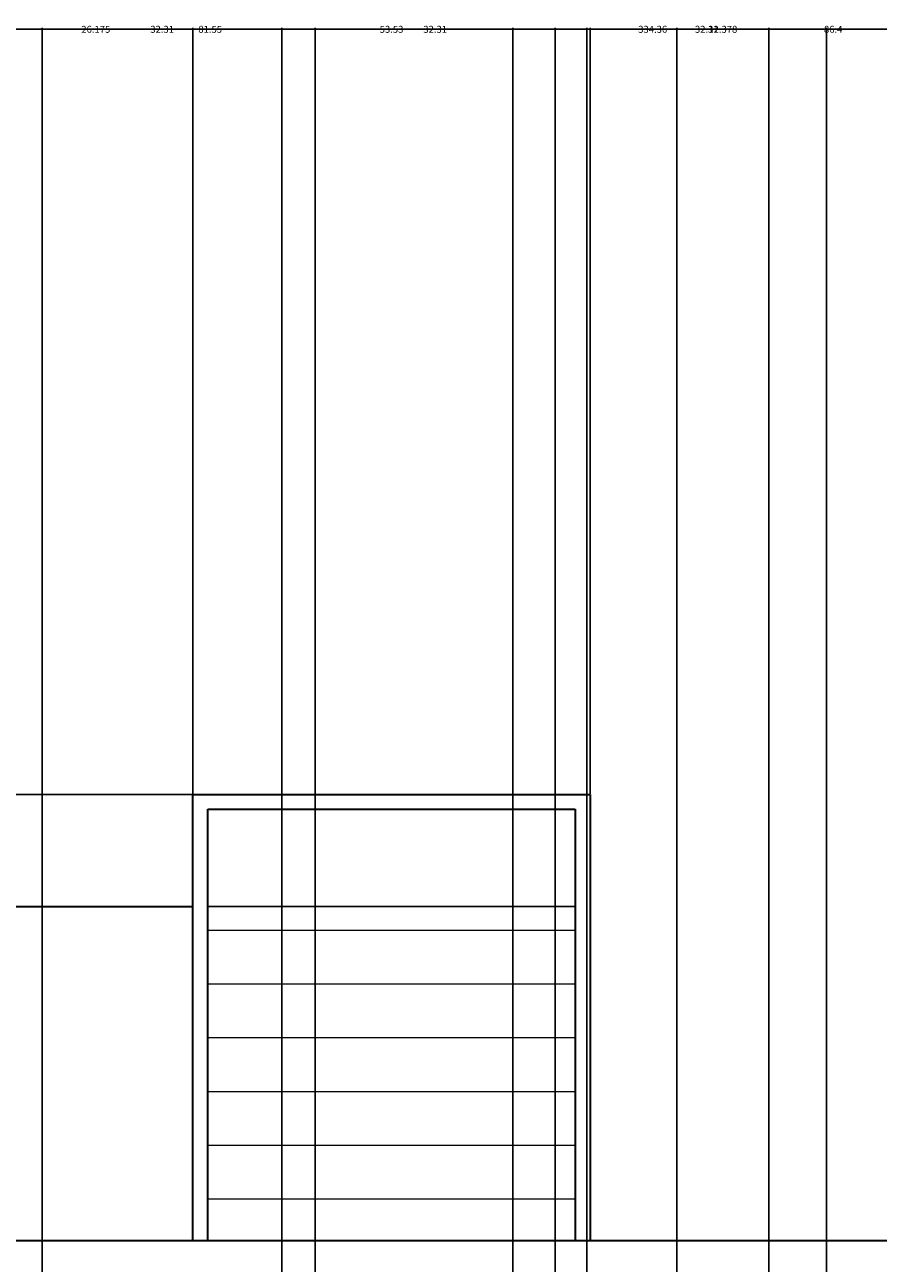
# Model space of a CAD drawing. Units: inches. Extents: x -5 to 714, y 84 to 644.
# Tile 14 of 20: x 342 to 457, y 477 to 644. Entities that reach past the tile are written whole.
import ezdxf

# ---------------------------------------------------------------- set-up
doc = ezdxf.new("R2010")
doc.units = ezdxf.units.IN
doc.header["$MEASUREMENT"] = 0
for name, color, linetype, lineweight in [('A-ANNO-DIMS', 2, 'Continuous', 18), ('A-ELEV', 7, 'Continuous', 35), ('A-ELEV-PATT', 8, 'Continuous', 13), ('A-GLAZ', 3, 'Continuous', 25)]:
    doc.layers.add(name, color=color, linetype=linetype, lineweight=lineweight)
doc.styles.get("Standard").update_dxf_attribs({"font": 'arial.ttf'})
doc.dimstyles.get("Standard").update_dxf_attribs({"dimtxt": 0.9375, "dimasz": 0.18, "dimexe": 0.18, "dimexo": 0.0625, "dimgap": 0.09, "dimtad": 0, "dimtih": 1, "dimtoh": 1, "dimdec": 4, "dimzin": 0, "dimdsep": 46, "dimlunit": 4, "dimtxsty": 'Standard', "dimcen": 0.09, "dimadec": 0, "dimazin": 0, "dimtfac": 1, "dimtdec": 4, "dimtofl": 0, "dimtmove": 0, "dimatfit": 3, "dimfxl": 1, "dimtolj": 1, "dimtzin": 0, "dimarcsym": 0})

# ---------------------------------------------------------------- blocks, each defined once
blk = doc.blocks.new('*D14')
at = {"layer": 'A-ANNO-DIMS', "color": 0, "lineweight": -2, "transparency": 16777216}
for p, q in [((338.11, 525.26), (338.11, 643.61)), ((338.29, 643.43), (349.15, 643.43)), ((364.1, 643.43), (353.24, 643.43)), ((364.28, 525.26), (364.28, 643.61))]:
    blk.add_line(p, q, dxfattribs=at)
at = {"layer": 'A-ANNO-DIMS', "color": 0, "transparency": 16777216}
for points in [[(338.29, 643.46), (338.29, 643.4), (338.11, 643.43)], [(364.1, 643.46), (364.1, 643.4), (364.28, 643.43)]]:
    blk.add_solid(points, dxfattribs=at)
at = {"layer": 'Defpoints', "color": 0, "transparency": 16777216}
for p in [(364.28, 643.43), (338.11, 525.19), (364.28, 525.19)]:
    blk.add_point(p, dxfattribs=at)
at = {"layer": 'A-ANNO-DIMS', "color": 0, "transparency": 16777216, "insert": (351.19, 643.43), "char_height": 0.938, "attachment_point": 5}
blk.add_mtext('\\A1;26.175', dxfattribs=at)
blk = doc.blocks.new('*D15')
at = {"layer": 'A-ANNO-DIMS', "color": 0, "lineweight": -2, "transparency": 16777216}
for p, q in [((364.28, 540.35), (364.28, 643.61)), ((364.46, 643.43), (389.37, 643.43)), ((417.63, 643.43), (392.72, 643.43)), ((417.81, 540.35), (417.81, 643.61))]:
    blk.add_line(p, q, dxfattribs=at)
at = {"layer": 'A-ANNO-DIMS', "color": 0, "transparency": 16777216}
for points in [[(364.46, 643.46), (364.46, 643.4), (364.28, 643.43)], [(417.63, 643.46), (417.63, 643.4), (417.81, 643.43)]]:
    blk.add_solid(points, dxfattribs=at)
at = {"layer": 'Defpoints', "color": 0, "transparency": 16777216}
for p in [(417.81, 643.43), (364.28, 540.29), (417.81, 540.29)]:
    blk.add_point(p, dxfattribs=at)
at = {"layer": 'A-ANNO-DIMS', "color": 0, "transparency": 16777216, "insert": (391.05, 643.43), "char_height": 0.938, "attachment_point": 5}
blk.add_mtext('\\A1;53.53', dxfattribs=at)
blk = doc.blocks.new('*D16')
at = {"layer": 'A-ANNO-DIMS', "color": 0, "lineweight": -2, "transparency": 16777216}
for p, q in [((364.22, 540.29), (-2.74, 540.29)), ((-2.56, 540.11), (-2.56, 510.8)), ((-2.56, 480.35), (-2.56, 509.66)), ((364.22, 480.17), (-2.74, 480.17))]:
    blk.add_line(p, q, dxfattribs=at)
at = {"layer": 'A-ANNO-DIMS', "color": 0, "transparency": 16777216}
for points in [[(-2.59, 540.11), (-2.53, 540.11), (-2.56, 540.29)], [(-2.59, 480.35), (-2.53, 480.35), (-2.56, 480.17)]]:
    blk.add_solid(points, dxfattribs=at)
at = {"layer": 'Defpoints', "color": 0, "transparency": 16777216}
for p in [(-2.56, 540.29), (364.28, 540.29), (364.28, 480.17)]:
    blk.add_point(p, dxfattribs=at)
at = {"layer": 'A-ANNO-DIMS', "color": 0, "transparency": 16777216, "insert": (-2.56, 510.23), "char_height": 0.938, "attachment_point": 5}
blk.add_mtext('\\A1;60.11', dxfattribs=at)
blk = doc.blocks.new('*D24')
at = {"layer": 'A-ANNO-DIMS', "color": 0, "lineweight": -2, "transparency": 16777216}
for p, q in [((126.73, 480.23), (126.73, 643.61)), ((126.91, 643.43), (295.25, 643.43)), ((466.92, 643.43), (298.58, 643.43)), ((467.1, 480.23), (467.1, 643.61))]:
    blk.add_line(p, q, dxfattribs=at)
at = {"layer": 'A-ANNO-DIMS', "color": 0, "transparency": 16777216}
for points in [[(126.91, 643.46), (126.91, 643.4), (126.73, 643.43)], [(466.92, 643.46), (466.92, 643.4), (467.1, 643.43)]]:
    blk.add_solid(points, dxfattribs=at)
at = {"layer": 'Defpoints', "color": 0, "transparency": 16777216}
for p in [(467.1, 643.43), (126.73, 480.17), (467.1, 480.17)]:
    blk.add_point(p, dxfattribs=at)
at = {"layer": 'A-ANNO-DIMS', "color": 0, "transparency": 16777216, "insert": (296.91, 643.43), "char_height": 0.938, "attachment_point": 5}
blk.add_mtext('\\A1;340.4', dxfattribs=at)
blk = doc.blocks.new('*D30')
at = {"layer": 'A-ANNO-DIMS', "color": 0, "lineweight": -2, "transparency": 16777216}
for p, q in [((429.51, 402.54), (429.51, 643.61)), ((429.69, 643.43), (433.71, 643.43)), ((441.71, 643.43), (437.69, 643.43)), ((441.89, 402.54), (441.89, 643.61))]:
    blk.add_line(p, q, dxfattribs=at)
at = {"layer": 'A-ANNO-DIMS', "color": 0, "transparency": 16777216}
for points in [[(429.69, 643.46), (429.69, 643.4), (429.51, 643.43)], [(441.71, 643.46), (441.71, 643.4), (441.89, 643.43)]]:
    blk.add_solid(points, dxfattribs=at)
at = {"layer": 'Defpoints', "color": 0, "transparency": 16777216}
for p in [(441.89, 643.43), (429.51, 402.48), (441.89, 402.48)]:
    blk.add_point(p, dxfattribs=at)
at = {"layer": 'A-ANNO-DIMS', "color": 0, "transparency": 16777216, "insert": (435.7, 643.43), "char_height": 0.938, "attachment_point": 5}
blk.add_mtext('\\A1;12.378', dxfattribs=at)
blk = doc.blocks.new('*D54')
at = {"layer": 'A-ANNO-DIMS', "color": 0, "lineweight": -2, "transparency": 16777216}
for p, q in [((259.07, 315.16), (259.07, 643.61)), ((259.25, 643.43), (424.21, 643.43)), ((593.25, 643.43), (428.28, 643.43)), ((593.43, 315.16), (593.43, 643.61))]:
    blk.add_line(p, q, dxfattribs=at)
at = {"layer": 'A-ANNO-DIMS', "color": 0, "transparency": 16777216}
for points in [[(259.25, 643.46), (259.25, 643.4), (259.07, 643.43)], [(593.25, 643.46), (593.25, 643.4), (593.43, 643.43)]]:
    blk.add_solid(points, dxfattribs=at)
at = {"layer": 'Defpoints', "color": 0, "transparency": 16777216}
for p in [(593.43, 643.43), (259.07, 315.1), (593.43, 315.1)]:
    blk.add_point(p, dxfattribs=at)
at = {"layer": 'A-ANNO-DIMS', "color": 0, "transparency": 16777216, "insert": (426.25, 643.43), "char_height": 0.938, "attachment_point": 5}
blk.add_mtext('\\A1;334.36', dxfattribs=at)
blk = doc.blocks.new('*D61')
at = {"layer": 'A-ANNO-DIMS', "color": 0, "lineweight": -2, "transparency": 16777216}
for p, q in [((325.83, 266.06), (325.83, 643.61)), ((326.01, 643.43), (364.93, 643.43)), ((407.2, 643.43), (368.28, 643.43)), ((407.38, 266.06), (407.38, 643.61))]:
    blk.add_line(p, q, dxfattribs=at)
at = {"layer": 'A-ANNO-DIMS', "color": 0, "transparency": 16777216}
for points in [[(326.01, 643.46), (326.01, 643.4), (325.83, 643.43)], [(407.2, 643.46), (407.2, 643.4), (407.38, 643.43)]]:
    blk.add_solid(points, dxfattribs=at)
at = {"layer": 'Defpoints', "color": 0, "transparency": 16777216}
for p in [(407.38, 643.43), (325.83, 266), (407.38, 266)]:
    blk.add_point(p, dxfattribs=at)
at = {"layer": 'A-ANNO-DIMS', "color": 0, "transparency": 16777216, "insert": (366.61, 643.43), "char_height": 0.938, "attachment_point": 5}
blk.add_mtext('\\A1;81.55', dxfattribs=at)
blk = doc.blocks.new('*D62')
at = {"layer": 'A-ANNO-DIMS', "color": 0, "lineweight": -2, "transparency": 16777216}
for p, q in [((407.38, 266.06), (407.38, 643.61)), ((407.56, 643.43), (449.27, 643.43)), ((493.6, 643.43), (451.89, 643.43)), ((493.78, 266.06), (493.78, 643.61))]:
    blk.add_line(p, q, dxfattribs=at)
at = {"layer": 'A-ANNO-DIMS', "color": 0, "transparency": 16777216}
for points in [[(407.56, 643.46), (407.56, 643.4), (407.38, 643.43)], [(493.6, 643.46), (493.6, 643.4), (493.78, 643.43)]]:
    blk.add_solid(points, dxfattribs=at)
at = {"layer": 'Defpoints', "color": 0, "transparency": 16777216}
for p in [(493.78, 643.43), (407.38, 266), (493.78, 266)]:
    blk.add_point(p, dxfattribs=at)
at = {"layer": 'A-ANNO-DIMS', "color": 0, "transparency": 16777216, "insert": (450.58, 643.43), "char_height": 0.938, "attachment_point": 5}
blk.add_mtext('\\A1;86.4', dxfattribs=at)
blk = doc.blocks.new('*D84')
at = {"layer": 'A-ANNO-DIMS', "color": 0, "lineweight": -2, "transparency": 16777216}
for p, q in [((343.97, 144.93), (343.97, 643.61)), ((344.15, 643.43), (358.54, 643.43)), ((376.1, 643.43), (361.71, 643.43)), ((376.28, 144.93), (376.28, 643.61))]:
    blk.add_line(p, q, dxfattribs=at)
at = {"layer": 'A-ANNO-DIMS', "color": 0, "transparency": 16777216}
for points in [[(344.15, 643.46), (344.15, 643.4), (343.97, 643.43)], [(376.1, 643.46), (376.1, 643.4), (376.28, 643.43)]]:
    blk.add_solid(points, dxfattribs=at)
at = {"layer": 'Defpoints', "color": 0, "transparency": 16777216}
for p in [(376.28, 643.43), (343.97, 144.86), (376.28, 144.86)]:
    blk.add_point(p, dxfattribs=at)
at = {"layer": 'A-ANNO-DIMS', "color": 0, "transparency": 16777216, "insert": (360.13, 643.43), "char_height": 0.938, "attachment_point": 5}
blk.add_mtext('\\A1;32.31', dxfattribs=at)
blk = doc.blocks.new('*D85')
at = {"layer": 'A-ANNO-DIMS', "color": 0, "lineweight": -2, "transparency": 16777216}
for p, q in [((380.78, 144.93), (380.78, 643.61)), ((380.96, 643.43), (395.35, 643.43)), ((412.91, 643.43), (398.51, 643.43)), ((413.09, 144.93), (413.09, 643.61))]:
    blk.add_line(p, q, dxfattribs=at)
at = {"layer": 'A-ANNO-DIMS', "color": 0, "transparency": 16777216}
for points in [[(380.96, 643.46), (380.96, 643.4), (380.78, 643.43)], [(412.91, 643.46), (412.91, 643.4), (413.09, 643.43)]]:
    blk.add_solid(points, dxfattribs=at)
at = {"layer": 'Defpoints', "color": 0, "transparency": 16777216}
for p in [(413.09, 643.43), (380.78, 144.86), (413.09, 144.86)]:
    blk.add_point(p, dxfattribs=at)
at = {"layer": 'A-ANNO-DIMS', "color": 0, "transparency": 16777216, "insert": (396.93, 643.43), "char_height": 0.938, "attachment_point": 5}
blk.add_mtext('\\A1;32.31', dxfattribs=at)
blk = doc.blocks.new('*D86')
at = {"layer": 'A-ANNO-DIMS', "color": 0, "lineweight": -2, "transparency": 16777216}
for p, q in [((417.38, 144.93), (417.38, 643.61)), ((417.56, 643.43), (431.96, 643.43)), ((449.51, 643.43), (435.12, 643.43)), ((449.69, 144.93), (449.69, 643.61))]:
    blk.add_line(p, q, dxfattribs=at)
at = {"layer": 'A-ANNO-DIMS', "color": 0, "transparency": 16777216}
for points in [[(417.56, 643.46), (417.56, 643.4), (417.38, 643.43)], [(449.51, 643.46), (449.51, 643.4), (449.69, 643.43)]]:
    blk.add_solid(points, dxfattribs=at)
at = {"layer": 'Defpoints', "color": 0, "transparency": 16777216}
for p in [(449.69, 643.43), (417.38, 144.86), (449.69, 144.86)]:
    blk.add_point(p, dxfattribs=at)
at = {"layer": 'A-ANNO-DIMS', "color": 0, "transparency": 16777216, "insert": (433.54, 643.43), "char_height": 0.938, "attachment_point": 5}
blk.add_mtext('\\A1;32.31', dxfattribs=at)

msp = doc.modelspace()

# ---------------------------------------------------------------- hatches: boundary and pattern name
at = {"layer": 'A-ELEV-PATT', "transparency": 33554687}
h = msp.add_hatch(dxfattribs=at)
h.set_pattern_fill('ANSI31', color=256, scale=58, angle=135)
h.paths.add_polyline_path([(249.4181, 345.1928), (237.2654, 345.1928), (200.7361, 345.1928), (200.7361, 201.1928), (249.4181, 201.1928)])
h.paths.add_polyline_path([(261.4349, 199.1928), (189.6349, 199.1928), (189.6349, 154.1176), (261.4349, 154.1176)])
h.paths.add_polyline_path([(415.8092, 525.1928), (366.2809, 525.1928), (366.2809, 480.1709), (415.8092, 480.1709)])

# ---------------------------------------------------------------- linework, layer by layer
at = {"layer": 'A-ELEV'}
for p, q in [((364.2809, 480.1709), (364.2809, 540.2857)), ((364.2809, 540.2857), (417.8092, 540.2857)), ((417.8092, 540.2857), (417.8092, 480.1709)), ((366.2809, 538.2857), (415.8092, 538.2857)), ((366.2809, 480.1709), (366.2809, 538.2857)), ((415.8092, 538.2857), (415.8092, 480.1709)), ((229.3575, 525.1928), (364.2809, 525.1928)), ((229.3575, 480.1709), (467.0994, 480.1709))]:
    msp.add_line(p, q, dxfattribs=at)
at = {"layer": 'A-GLAZ'}
msp.add_lwpolyline([(366.2809, 525.1928), (415.8092, 525.1928), (415.8092, 480.1709), (366.2809, 480.1709)], close=True, dxfattribs=at)

# ---------------------------------------------------------------- dimensions: what is measured, and where the dimension line sits
at = {"layer": 'A-ANNO-DIMS'}
for base, p1, p2, override, picture, middle in [((467.0994, 643.4276), (126.7303, 480.1709), (467.0994, 480.1709), {"dimdec": 1, "dimlfac": 1, "dimrnd": 0, "dimzin": 0, "dimdsep": 46, "dimlunit": 2}, '*D24', (296.9148, 643.4276)), ((593.428, 643.4276), (259.0665, 315.0968), (593.428, 315.0968), {"dimdec": 2, "dimlfac": 1, "dimrnd": 0, "dimzin": 0, "dimdsep": 46, "dimlunit": 2}, '*D54', (426.2472, 643.4276)), ((407.3813, 643.4276), (325.8305, 266.0021), (407.3813, 266.0021), {"dimdec": 2, "dimlfac": 1, "dimrnd": 0, "dimzin": 0, "dimdsep": 46, "dimlunit": 2}, '*D61', (366.6059, 643.4276)), ((364.2809, 643.4276), (338.106, 525.1928), (364.2809, 525.1928), {"dimdec": 3, "dimlfac": 1, "dimrnd": 0, "dimzin": 0, "dimdsep": 46, "dimlunit": 2}, '*D14', (351.1934, 643.4276)), ((376.2796, 643.4276), (343.9704, 144.8639), (376.2796, 144.8639), {"dimdec": 2, "dimlfac": 1, "dimrnd": 0, "dimzin": 0, "dimdsep": 46, "dimlunit": 2}, '*D84', (360.125, 643.4276)), ((417.8092, 643.4276), (364.2809, 540.2857), (417.8092, 540.2857), {"dimdec": 2, "dimlfac": 1, "dimrnd": 0, "dimzin": 0, "dimdsep": 46, "dimlunit": 2}, '*D15', (391.0451, 643.4276)), ((413.0876, 643.4276), (380.7784, 144.8639), (413.0876, 144.8639), {"dimdec": 2, "dimlfac": 1, "dimrnd": 0, "dimzin": 0, "dimdsep": 46, "dimlunit": 2}, '*D85', (396.933, 643.4276)), ((493.7771, 643.4276), (407.3813, 266.0021), (493.7771, 266.0021), {"dimdec": 1, "dimlfac": 1, "dimrnd": 0, "dimzin": 0, "dimdsep": 46, "dimlunit": 2}, '*D62', (450.5792, 643.4276)), ((449.6911, 643.4276), (417.3818, 144.8639), (449.6911, 144.8639), {"dimdec": 2, "dimlfac": 1, "dimrnd": 0, "dimzin": 0, "dimdsep": 46, "dimlunit": 2}, '*D86', (433.5365, 643.4276)), ((441.8872, 643.4276), (429.5094, 402.4806), (441.8872, 402.4806), {"dimdec": 3, "dimlfac": 1, "dimrnd": 0, "dimzin": 0, "dimdsep": 46, "dimlunit": 2}, '*D30', (435.6983, 643.4276))]:
    dim = msp.add_linear_dim(base=base, p1=p1, p2=p2, dimstyle='Standard', override=override, dxfattribs=at)
    dim.commit()
    dim.dimension.update_dxf_attribs({"geometry": picture, "text_midpoint": middle})
dim = msp.add_linear_dim(base=(-2.5605, 540.2857), p1=(364.2809, 480.1709), p2=(364.2809, 540.2857), angle=90, dimstyle='Standard', override={"dimdec": 2, "dimlfac": 1, "dimrnd": 0, "dimzin": 0, "dimdsep": 46, "dimlunit": 2}, dxfattribs=at)
dim.commit()
dim.dimension.update_dxf_attribs({"geometry": '*D16', "text_midpoint": (-2.5605, 510.2283)})

doc.saveas('drawing.dxf')
